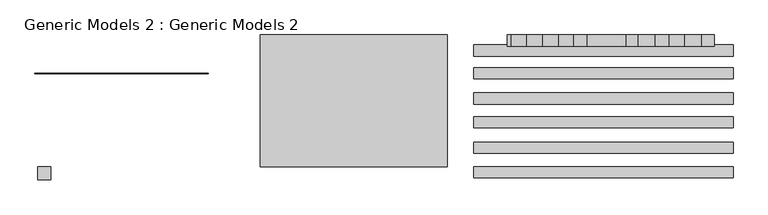
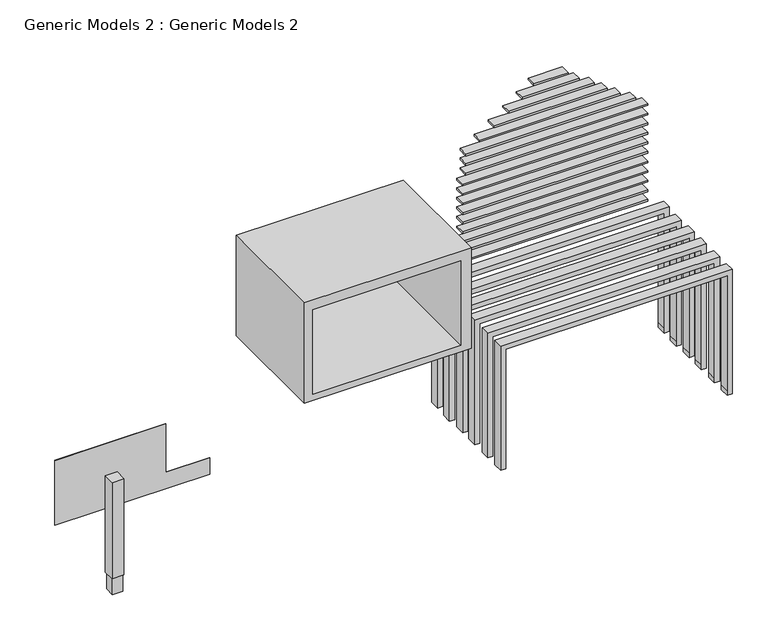
"""IFC4 building model written with IfcOpenShell, lengths in millimetres: proxy geometry, Generic Models 2 : Generic Models 2."""

from ifc_helpers import new_model, si_unit, frame, origin, origin_with_axes, place, context, project, spatial, polyline, outline, extrude, source, transform, mapped, element, save


def generic_models_2_generic_models_2_f6a97bfe(model_context):
    return source(origin(), model_context, "Body", "SweptSolid", [
        extrude(outline(polyline([(2559.6753529, -1658.0111529), (1524.6253529, -1658.0111529), (1524.6253529, -1353.2111529), (2559.6753529, -1353.2111529), (2559.6753529, -1658.0111529)])), frame((0.0, 0.0, 8887.9910655), z_axis=(0.0, 0.0, 1.0), x_axis=(1.0, 0.0, 0.0)), (0.0, 0.0, 1.0), 57.15),
        extrude(outline(polyline([(2889.8753529, -1658.0111529), (1169.0253529, -1658.0111529), (1169.0253529, -1353.2111529), (2889.8753529, -1353.2111529), (2889.8753529, -1658.0111529)])), frame((0.0, 0.0, 8583.1910655), z_axis=(0.0, 0.0, 1.0), x_axis=(1.0, 0.0, 0.0)), (0.0, 0.0, 1.0), 57.15),
        extrude(outline(polyline([(3347.0753529, -1658.0111529), (762.6253529, -1658.0111529), (762.6253529, -1353.2111529), (3347.0753529, -1353.2111529), (3347.0753529, -1658.0111529)])), frame((0.0, 0.0, 8278.3910655), z_axis=(0.0, 0.0, 1.0), x_axis=(1.0, 0.0, 0.0)), (0.0, 0.0, 1.0), 57.15),
        extrude(outline(polyline([(3728.0753529, -1658.0111529), (330.8253529, -1658.0111529), (330.8253529, -1353.2111529), (3728.0753529, -1353.2111529), (3728.0753529, -1658.0111529)])), frame((0.0, 0.0, 7973.5910655), z_axis=(0.0, 0.0, 1.0), x_axis=(1.0, 0.0, 0.0)), (0.0, 0.0, 1.0), 57.15),
        extrude(outline(polyline([(4134.4753529, -1658.0111529), (-100.9746471, -1658.0111529), (-100.9746471, -1353.2111529), (4134.4753529, -1353.2111529), (4134.4753529, -1658.0111529)])), frame((0.0, 0.0, 7668.7910655), z_axis=(0.0, 0.0, 1.0), x_axis=(1.0, 0.0, 0.0)), (0.0, 0.0, 1.0), 57.15),
        extrude(outline(polyline([(4596.4705989, -1658.0111529), (-521.6294011, -1658.0111529), (-521.6294011, -1353.2111529), (4596.4705989, -1353.2111529), (4596.4705989, -1658.0111529)])), frame((0.0, 0.0, 7363.9910655), z_axis=(0.0, 0.0, 1.0), x_axis=(1.0, 0.0, 0.0)), (0.0, 0.0, 1.0), 57.15),
        extrude(outline(polyline([(4952.0705989, -1658.0111529), (-521.6294011, -1658.0111529), (-521.6294011, -1353.2111529), (4952.0705989, -1353.2111529), (4952.0705989, -1658.0111529)])), frame((0.0, 0.0, 7059.1910655), z_axis=(0.0, 0.0, 1.0), x_axis=(1.0, 0.0, 0.0)), (0.0, 0.0, 1.0), 57.15),
        extrude(outline(polyline([(4952.0705989, -1658.0111529), (-521.6294011, -1658.0111529), (-521.6294011, -1353.2111529), (4952.0705989, -1353.2111529), (4952.0705989, -1658.0111529)])), frame((0.0, 0.0, 6754.3910655), z_axis=(0.0, 0.0, 1.0), x_axis=(1.0, 0.0, 0.0)), (0.0, 0.0, 1.0), 57.15),
        extrude(outline(polyline([(4952.0705989, -1658.0111529), (-623.2294011, -1658.0111529), (-623.2294011, -1353.2111529), (4952.0705989, -1353.2111529), (4952.0705989, -1658.0111529)])), frame((0.0, 0.0, 6449.5910655), z_axis=(0.0, 0.0, 1.0), x_axis=(1.0, 0.0, 0.0)), (0.0, 0.0, 1.0), 57.15),
        extrude(outline(polyline([(4952.0705989, -1658.0111529), (-623.2294011, -1658.0111529), (-623.2294011, -1353.2111529), (4952.0705989, -1353.2111529), (4952.0705989, -1658.0111529)])), frame((0.0, 0.0, 6144.7910655), z_axis=(0.0, 0.0, 1.0), x_axis=(1.0, 0.0, 0.0)), (0.0, 0.0, 1.0), 57.15),
        extrude(outline(polyline([(4952.0705989, -1658.0111529), (-623.2294011, -1658.0111529), (-623.2294011, -1353.2111529), (4952.0705989, -1353.2111529), (4952.0705989, -1658.0111529)])), frame((0.0, 0.0, 5839.9910655), z_axis=(0.0, 0.0, 1.0), x_axis=(1.0, 0.0, 0.0)), (0.0, 0.0, 1.0), 57.15),
        extrude(outline(polyline([(4952.0705989, -1658.0111529), (-623.2294011, -1658.0111529), (-623.2294011, -1353.2111529), (4952.0705989, -1353.2111529), (4952.0705989, -1658.0111529)])), frame((0.0, 0.0, 5535.1910655), z_axis=(0.0, 0.0, 1.0), x_axis=(1.0, 0.0, 0.0)), (0.0, 0.0, 1.0), 57.15),
        extrude(outline(polyline([(4952.0705989, -1658.0111529), (-623.2294011, -1658.0111529), (-623.2294011, -1353.2111529), (4952.0705989, -1353.2111529), (4952.0705989, -1658.0111529)])), frame((0.0, 0.0, 5230.3910655), z_axis=(0.0, 0.0, 1.0), x_axis=(1.0, 0.0, 0.0)), (0.0, 0.0, 1.0), 57.15),
        extrude(outline(polyline([(4952.0705989, -1658.0111529), (-623.2294011, -1658.0111529), (-623.2294011, -1353.2111529), (4952.0705989, -1353.2111529), (4952.0705989, -1658.0111529)])), frame((0.0, 0.0, 4925.5910655), z_axis=(0.0, 0.0, 1.0), x_axis=(1.0, 0.0, 0.0)), (0.0, 0.0, 1.0), 57.15),
        extrude(outline(polyline([(4952.0705989, -1658.0111529), (-623.2294011, -1658.0111529), (-623.2294011, -1353.2111529), (4952.0705989, -1353.2111529), (4952.0705989, -1658.0111529)])), frame((0.0, 0.0, 4620.7910655), z_axis=(0.0, 0.0, 1.0), x_axis=(1.0, 0.0, 0.0)), (0.0, 0.0, 1.0), 57.15),
        extrude(outline(polyline([(4952.0705989, -1658.0111529), (-623.2294011, -1658.0111529), (-623.2294011, -1353.2111529), (4952.0705989, -1353.2111529), (4952.0705989, -1658.0111529)])), frame((0.0, 0.0, 4315.9910655), z_axis=(0.0, 0.0, 1.0), x_axis=(1.0, 0.0, 0.0)), (0.0, 0.0, 1.0), 57.15),
        extrude(outline(polyline([(4952.0705989, -1658.0111529), (-623.2294011, -1658.0111529), (-623.2294011, -1353.2111529), (4952.0705989, -1353.2111529), (4952.0705989, -1658.0111529)])), frame((0.0, 0.0, 4011.1910655), z_axis=(0.0, 0.0, 1.0), x_axis=(1.0, 0.0, 0.0)), (0.0, 0.0, 1.0), 57.15),
        extrude(outline(polyline([(3657.6, -1372.5294011), (3657.6, 5301.3607112), (0.0, 5301.3607112), (-152.4, 5301.3607112), (-152.4, 5453.7607112), (3810.0, 5453.7607112), (3810.0, -1524.9294011), (-152.4, -1524.9294011), (-152.4, -1372.5294011), (0.0, -1372.5294011), (3657.6, -1372.5294011)])), frame((0.0, -1924.7111529, 0.0), z_axis=(0.0, 1.0, 0.0), x_axis=(0.0, 0.0, 1.0)), (0.0, 0.0, 1.0), 304.8),
        extrude(outline(polyline([(3606.8, -1372.5294011), (3606.8, 5301.3607112), (-50.8, 5301.3607112), (-203.2, 5301.3607112), (-203.2, 5453.7607112), (3759.2, 5453.7607112), (3759.2, -1524.9294011), (-203.2, -1524.9294011), (-203.2, -1372.5294011), (-50.8, -1372.5294011), (3606.8, -1372.5294011)])), frame((0.0, -2534.3111529, 0.0), z_axis=(0.0, 1.0, 0.0), x_axis=(0.0, 0.0, 1.0)), (0.0, 0.0, 1.0), 304.8),
        extrude(outline(polyline([(3657.6, -1372.5294011), (3657.6, 5301.3607112), (0.0, 5301.3607112), (-152.4, 5301.3607112), (-152.4, 5453.7607112), (3810.0, 5453.7607112), (3810.0, -1524.9294011), (-152.4, -1524.9294011), (-152.4, -1372.5294011), (0.0, -1372.5294011), (3657.6, -1372.5294011)])), frame((0.0, -3220.1111529, 0.0), z_axis=(0.0, 1.0, 0.0), x_axis=(0.0, 0.0, 1.0)), (0.0, 0.0, 1.0), 304.8),
        extrude(outline(polyline([(3657.6, -1372.5294011), (3657.6, 5301.3607112), (0.0, 5301.3607112), (-152.4, 5301.3607112), (-152.4, 5453.7607112), (3810.0, 5453.7607112), (3810.0, -1524.9294011), (-152.4, -1524.9294011), (-152.4, -1372.5294011), (0.0, -1372.5294011), (3657.6, -1372.5294011)])), frame((0.0, -3855.1111529, 0.0), z_axis=(0.0, 1.0, 0.0), x_axis=(0.0, 0.0, 1.0)), (0.0, 0.0, 1.0), 304.8),
        extrude(outline(polyline([(3657.6, -1372.5294011), (3657.6, 5301.3607112), (0.0, 5301.3607112), (-152.4, 5301.3607112), (-152.4, 5453.7607112), (3810.0, 5453.7607112), (3810.0, -1524.9294011), (-152.4, -1524.9294011), (-152.4, -1372.5294011), (0.0, -1372.5294011), (3657.6, -1372.5294011)])), frame((0.0, -4540.9111529, 0.0), z_axis=(0.0, 1.0, 0.0), x_axis=(0.0, 0.0, 1.0)), (0.0, 0.0, 1.0), 304.8),
        extrude(outline(polyline([(3657.6, -1372.5294011), (3657.6, 5301.3607112), (0.0, 5301.3607112), (-152.4, 5301.3607112), (-152.4, 5453.7607112), (3810.0, 5453.7607112), (3810.0, -1524.9294011), (-152.4, -1524.9294011), (-152.4, -1372.5294011), (0.0, -1372.5294011), (3657.6, -1372.5294011)])), frame((0.0, -5201.3111529, 0.0), z_axis=(0.0, 1.0, 0.0), x_axis=(0.0, 0.0, 1.0)), (0.0, 0.0, 1.0), 304.8),
        extrude(outline(polyline([(2590.8, -13335.9294011), (530.6554192, -13335.9294011), (530.6554192, -8675.0294011), (1047.6775384, -8675.0294011), (1047.6775384, -9995.8294011), (2590.8, -9995.8294011), (2590.8, -13335.9294011)])), frame((0.0, -2394.6111529, 0.0), z_axis=(0.0, 1.0, 0.0), x_axis=(0.0, 0.0, 1.0)), (0.0, 0.0, 1.0), 12.7),
        extrude(outline(polyline([(-13259.7294011, -4894.4534597), (-12904.1294011, -4894.4534597), (-12904.1294011, -5250.0534597), (-13259.7294011, -5250.0534597), (-13259.7294011, -4894.4534597)])), frame((0.0, 0.0, 530.6554192), z_axis=(0.0, 0.0, 1.0), x_axis=(1.0, 0.0, 0.0)), (0.0, 0.0, 1.0), 3068.032243),
        extrude(outline(polyline([(-13234.3294011, -5224.6534597), (-13234.3294011, -4919.8534597), (-12929.5294011, -4919.8534597), (-12929.5294011, -5224.6534597), (-13234.3294011, -5224.6534597)])), origin_with_axes(), (0.0, 0.0, 1.0), 530.6554192),
        extrude(outline(polyline([(7010.4, -2236.1294011), (7010.4, -7265.3294011), (3807.5858818, -7265.3294011), (3807.5858818, -2236.1294011), (7010.4, -2236.1294011)]), holes=[polyline([(6705.6, -2553.6294011), (4013.0501099, -2553.6294011), (4013.0501099, -7011.3294011), (6705.6, -7011.3294011), (6705.6, -2553.6294011)])]), frame((0.0, -4896.5111529, 0.0), z_axis=(0.0, 1.0, 0.0), x_axis=(0.0, 0.0, 1.0)), (0.0, 0.0, 1.0), 3543.3),
    ])


if __name__ == "__main__":
    model = new_model("IFC4")
    model_context = context("Model", 3, world=origin())
    ifc_project = project(units=[si_unit("LENGTHUNIT", "METRE", prefix="MILLI")], contexts=[model_context])
    site = spatial("IfcSite", under=ifc_project)
    building = spatial("IfcBuilding", under=site)
    placement = place(None, origin())
    generic_models_2_generic_models_2_shape = generic_models_2_generic_models_2_f6a97bfe(model_context)
    element("IfcBuildingElementProxy", 1, Name="Generic Models 2 : Generic Models 2", ObjectType="Generic Models 2 : Generic Models 2", at=placement, inside=building, context=model_context, shape_type="MappedRepresentation", body=[
        mapped(generic_models_2_generic_models_2_shape, transform((0.0, 0.0, 0.0), x_axis=(1.0, 0.0, 0.0), y_axis=(0.0, 1.0, 0.0), z_axis=(0.0, 0.0, 1.0))),
    ])
    save(model, "model.ifc")

# Revit data of these elements
# Element 1 (IfcBuildingElementProxy, "Generic Models 2 : Generic Models 2")
#   Materials on its faces: "Gypsum Wall Board", "tiles"
# Materials
#   "Gypsum Wall Board": class "Generic", colour RGB 127 127 127, transparency 0, Description = "Gypsum Wall Board", Cost = 0
#   "tiles": class "Generic", colour RGB 120 120 120, transparency 0, Cost = 0
